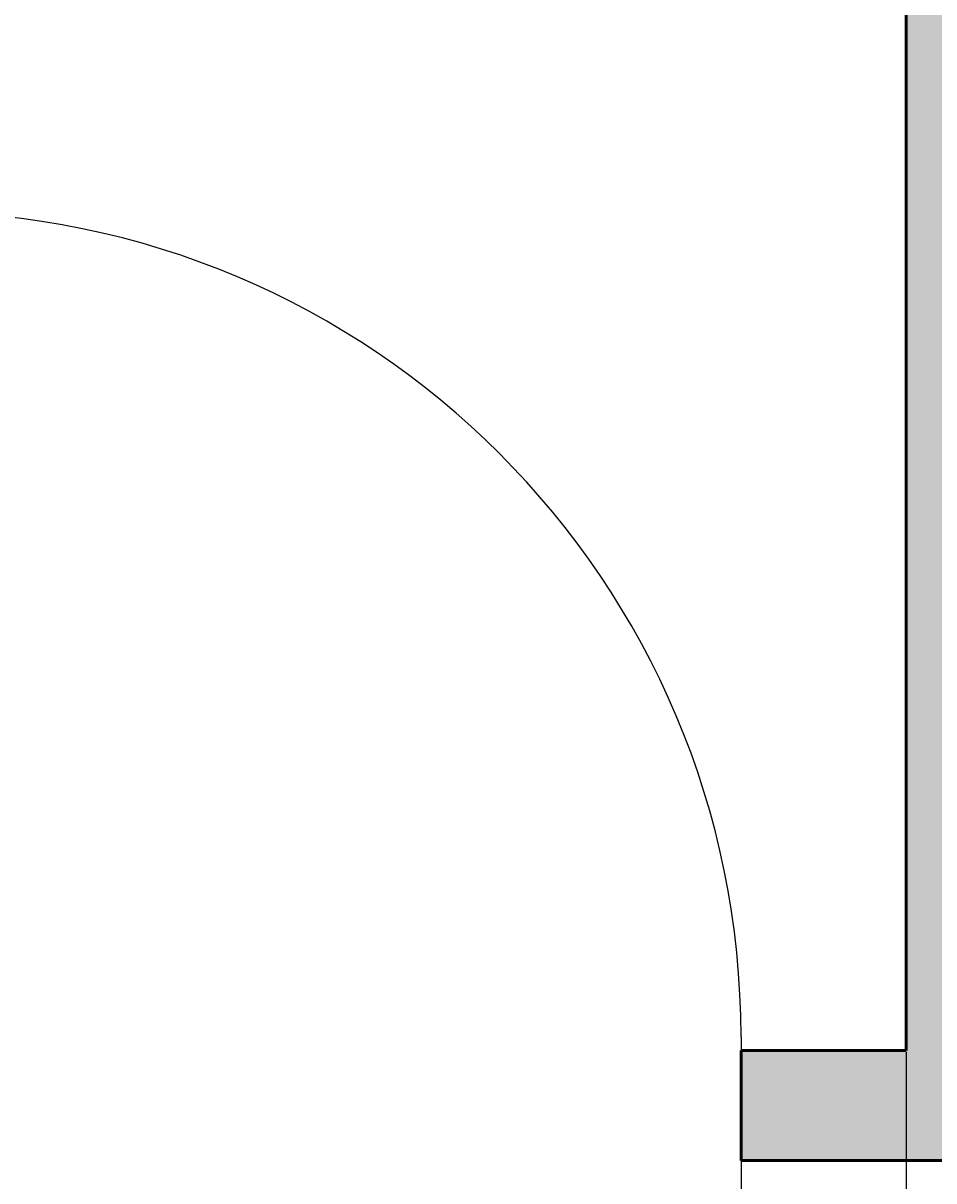
# Model space of a CAD drawing. Units: inches. Extents: x 2307 to 2544, y 2171 to 2540.
# Tile 21 of 52: x 2420 to 2453, y 2387 to 2429. Entities that reach past the tile are written whole.
import ezdxf

# ---------------------------------------------------------------- set-up
doc = ezdxf.new("R2010")
doc.units = ezdxf.units.IN
for name, color, linetype, lineweight in [('A-ANNO-DIMS', 2, 'Continuous', 18), ('A-DOOR', 3, 'Continuous', 25), ('A-WALL', 7, 'Continuous', 50)]:
    doc.layers.add(name, color=color, linetype=linetype, lineweight=lineweight)
doc.layers.add('A-WALL-PATT', color=18, linetype='Continuous', lineweight=13, true_color=0x000000)
doc.styles.get("Standard").update_dxf_attribs({"font": 'arial.ttf'})
doc.dimstyles.get("Standard").update_dxf_attribs({"dimtxt": 0.18, "dimasz": 0.18, "dimexe": 0.18, "dimexo": 0.0625, "dimgap": 0.09, "dimtad": 0, "dimtih": 1, "dimtoh": 1, "dimdec": 4, "dimzin": 0, "dimdsep": 46, "dimtxsty": 'Standard', "dimcen": 0.09, "dimadec": 0, "dimazin": 0, "dimtfac": 1, "dimtdec": 4, "dimtofl": 0, "dimtmove": 0, "dimatfit": 3, "dimfxl": 1, "dimtolj": 1, "dimtzin": 0, "dimarcsym": 0})

# ---------------------------------------------------------------- blocks, each defined once
blk = doc.blocks.new('*U13')
for p, q in [((0, 0), (0, -6)), ((40, 0), (40, -6))]:
    blk.add_line(p, q)
blk.add_lwpolyline([(0, 0), (0, 40), (1.75, 40), (1.75, 0)], close=True)
blk.add_arc((0, 0), 40, 0, 90)
blk = doc.blocks.new('*D51')
at = {"layer": 'A-ANNO-DIMS', "color": 0, "lineweight": -2, "transparency": 16777216}
for p, q in [((2415.696, 2387.447), (2415.696, 2368.18)), ((2445.696, 2387.447), (2445.696, 2368.18)), ((2415.876, 2368.36), (2430.477, 2368.36)), ((2445.516, 2368.36), (2430.914, 2368.36))]:
    blk.add_line(p, q, dxfattribs=at)
at = {"layer": 'A-ANNO-DIMS', "color": 0, "transparency": 16777216}
for points in [[(2415.876, 2368.39), (2415.876, 2368.33), (2415.696, 2368.36)], [(2445.516, 2368.39), (2445.516, 2368.33), (2445.696, 2368.36)]]:
    blk.add_solid(points, dxfattribs=at)
at = {"layer": 'Defpoints', "color": 0, "transparency": 16777216}
for p in [(2415.696, 2387.51), (2445.696, 2387.51), (2415.696, 2368.36)]:
    blk.add_point(p, dxfattribs=at)
at = {"layer": 'A-ANNO-DIMS', "color": 0, "transparency": 16777216, "insert": (2430.696, 2368.36), "char_height": 0.18, "attachment_point": 5}
blk.add_mtext('\\A1;30', dxfattribs=at)
blk = doc.blocks.new('*D52')
at = {"layer": 'A-ANNO-DIMS', "color": 0, "lineweight": -2, "transparency": 16777216}
for p, q in [((2445.696, 2391.447), (2445.696, 2372.18)), ((2451.696, 2391.447), (2451.696, 2372.18)), ((2445.876, 2372.36), (2448.546, 2372.36)), ((2451.516, 2372.36), (2448.845, 2372.36))]:
    blk.add_line(p, q, dxfattribs=at)
at = {"layer": 'A-ANNO-DIMS', "color": 0, "transparency": 16777216}
for points in [[(2445.876, 2372.39), (2445.876, 2372.33), (2445.696, 2372.36)], [(2451.516, 2372.39), (2451.516, 2372.33), (2451.696, 2372.36)]]:
    blk.add_solid(points, dxfattribs=at)
at = {"layer": 'Defpoints', "color": 0, "transparency": 16777216}
for p in [(2445.696, 2391.51), (2451.696, 2391.51), (2445.696, 2372.36)]:
    blk.add_point(p, dxfattribs=at)
at = {"layer": 'A-ANNO-DIMS', "color": 0, "transparency": 16777216, "insert": (2448.696, 2372.36), "char_height": 0.18, "attachment_point": 5}
blk.add_mtext('\\A1;6', dxfattribs=at)

msp = doc.modelspace()

# ---------------------------------------------------------------- hatches: boundary and pattern name
at = {"layer": 'A-WALL-PATT'}
h = msp.add_hatch(color=256, dxfattribs=at)
h.dxf.hatch_style = 1
h.paths.add_polyline_path([(2433.6935, 2199.5096), (2415.6423, 2199.5096), (2415.6423, 2190.5096), (2433.7832, 2190.5096)], flags=17)
h.paths.add_polyline_path([(2367.6423, 2199.5096), (2335.6958, 2199.5096), (2335.6958, 2307.3983), (2326.6958, 2307.3983), (2326.6958, 2190.5096), (2367.6423, 2190.5096)])
h.paths.add_polyline_path([(2524.6958, 2520.5096), (2496.7832, 2520.5096), (2496.7832, 2515.5149), (2472.7832, 2515.5149), (2472.7832, 2520.5096), (2415.4028, 2520.5096), (2415.4028, 2511.5096), (2451.6958, 2511.5096), (2451.6958, 2439.5096), (2451.6958, 2391.5096), (2445.6958, 2391.5096), (2445.6958, 2387.5096), (2455.6958, 2387.5096), (2455.6958, 2435.5096), (2461.6958, 2435.5096), (2461.6958, 2439.5096), (2455.6958, 2439.5096), (2455.6958, 2511.5096), (2515.6958, 2511.5096), (2515.6958, 2439.5096), (2491.6958, 2439.5096), (2491.6958, 2435.5096), (2515.6958, 2435.5096), (2515.6958, 2319.5096), (2451.6958, 2319.5096), (2451.6958, 2281.5096), (2481.6958, 2281.5096), (2481.6958, 2225.5096), (2485.6958, 2225.5096), (2485.6958, 2285.5096), (2455.6958, 2285.5096), (2455.6958, 2315.5096), (2515.6958, 2315.5096), (2515.6958, 2199.5096), (2469.6952, 2199.5096), (2469.785, 2190.5096), (2524.6958, 2190.5096)])

# ---------------------------------------------------------------- linework, layer by layer
at = {"layer": 'A-WALL'}
for p, q in [((2451.6958, 2391.5096), (2451.6958, 2511.5096)), ((2451.6958, 2435.5096), (2451.6958, 2391.5096)), ((2445.6958, 2391.5096), (2445.6958, 2387.5096)), ((2445.6958, 2391.5096), (2451.6958, 2391.5096)), ((2445.6958, 2387.5096), (2455.6958, 2387.5096))]:
    msp.add_line(p, q, dxfattribs=at)

# ---------------------------------------------------------------- block references
at = {"layer": 'A-DOOR', "xscale": 0.75, "yscale": 0.75, "zscale": 0.75}
msp.add_blockref('*U13', (2415.6958, 2392.0096), dxfattribs=at)

# ---------------------------------------------------------------- dimensions: what is measured, and where the dimension line sits
at = {"layer": 'A-ANNO-DIMS'}
for base, p1, p2, picture, middle in [((2445.6958, 2372.3596), (2451.6958, 2391.5096), (2445.6958, 2391.5096), '*D52', (2448.6958, 2372.3596)), ((2415.6958, 2368.3596), (2445.6958, 2387.5096), (2415.6958, 2387.5096), '*D51', (2430.6958, 2368.3596))]:
    dim = msp.add_linear_dim(base=base, p1=p1, p2=p2, angle=180, dimstyle='Standard', override={"dimdec": 0, "dimlfac": 1, "dimrnd": 0, "dimzin": 0, "dimdsep": 46, "dimlunit": 2}, dxfattribs=at)
    dim.commit()
    dim.dimension.update_dxf_attribs({"geometry": picture, "text_midpoint": middle})

doc.saveas('drawing.dxf')
